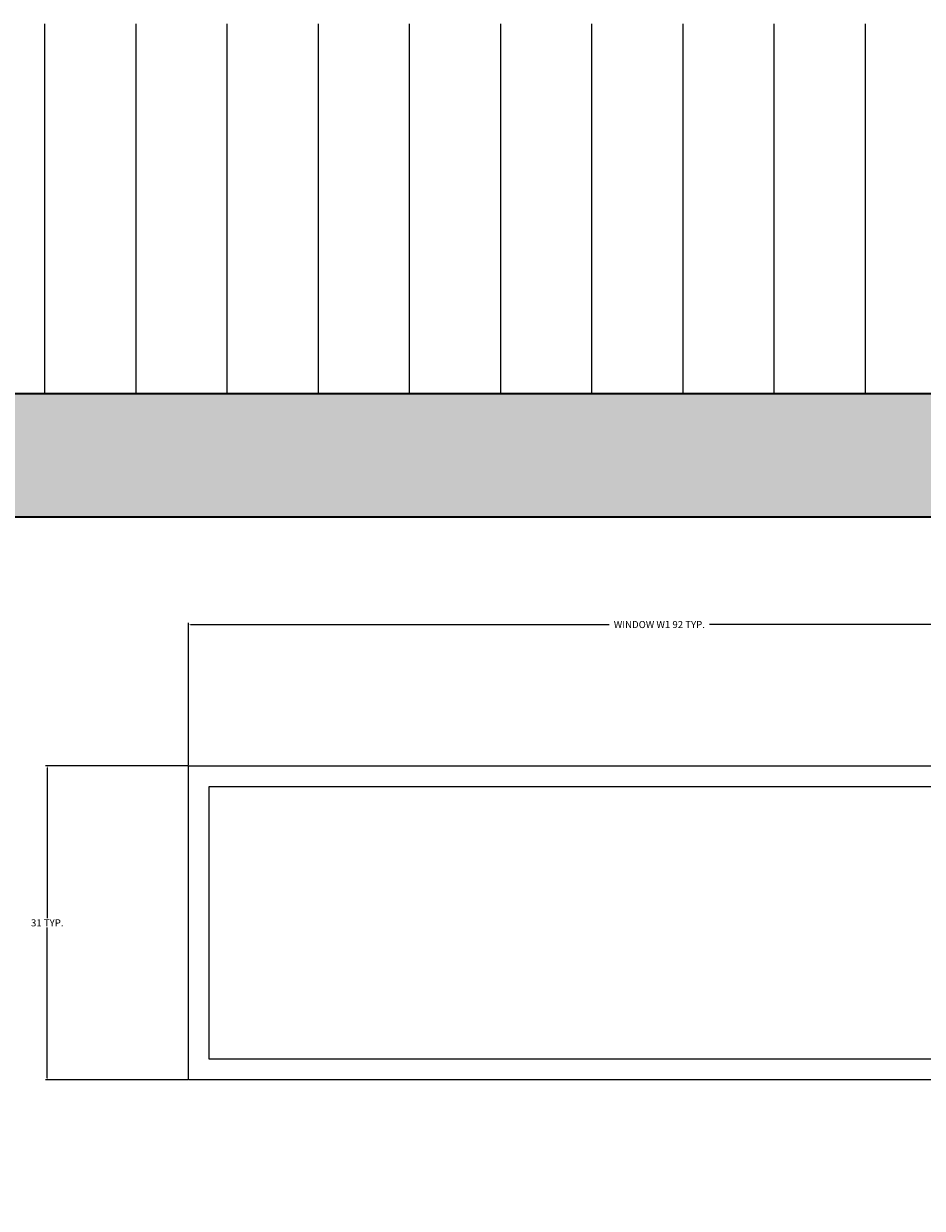
# Model space of a CAD drawing. Units: inches. Extents: x -145 to 510, y 5 to 386.
# Tile 23 of 25: x 335 to 423, y 157 to 272. Entities that reach past the tile are written whole.
import ezdxf

# ---------------------------------------------------------------- set-up
doc = ezdxf.new("R2010")
doc.units = ezdxf.units.IN
doc.header["$MEASUREMENT"] = 0
for name, color, linetype, lineweight in [('A-ANNO-DIMS', 2, 'Continuous', 18), ('A-ELEV', 7, 'Continuous', 35), ('A-ELEV-PATT', 8, 'Continuous', 13), ('A-GLAZ', 4, 'Continuous', 25)]:
    doc.layers.add(name, color=color, linetype=linetype, lineweight=lineweight)
doc.styles.get("Standard").update_dxf_attribs({"font": 'arial.ttf'})
doc.dimstyles.get("Standard").update_dxf_attribs({"dimtxt": 0.6875, "dimasz": 0.18, "dimexe": 0.18, "dimexo": 0.0625, "dimgap": 0.09, "dimtad": 0, "dimtih": 1, "dimtoh": 1, "dimdec": 4, "dimzin": 0, "dimdsep": 46, "dimlunit": 4, "dimtxsty": 'Standard', "dimcen": 0.09, "dimadec": 0, "dimazin": 0, "dimtfac": 1, "dimtdec": 4, "dimtofl": 0, "dimtmove": 0, "dimatfit": 3, "dimfxl": 1, "dimtolj": 1, "dimtzin": 0, "dimarcsym": 0})

# ---------------------------------------------------------------- blocks, each defined once
blk = doc.blocks.new('WIN-2200')
for points in [[(0, 30.55), (91.67, 30.55), (91.67, 0), (0, 0)], [(2, 28.55), (89.67, 28.55), (89.67, 2), (2, 2)]]:
    blk.add_lwpolyline(points, close=True)
blk = doc.blocks.new('*D5')
at = {"layer": 'A-ANNO-DIMS', "color": 0, "lineweight": -2, "transparency": 16777216}
for p, q in [((351.23, 199.73), (351.23, 213.6)), ((351.41, 213.42), (392.2, 213.42)), ((442.72, 213.42), (401.94, 213.42)), ((442.9, 199.73), (442.9, 213.6))]:
    blk.add_line(p, q, dxfattribs=at)
at = {"layer": 'A-ANNO-DIMS', "color": 0, "transparency": 16777216}
for points in [[(351.41, 213.45), (351.41, 213.39), (351.23, 213.42)], [(442.72, 213.45), (442.72, 213.39), (442.9, 213.42)]]:
    blk.add_solid(points, dxfattribs=at)
at = {"layer": 'Defpoints', "color": 0, "transparency": 16777216}
for p in [(442.9, 213.42), (351.23, 199.67), (442.9, 199.67)]:
    blk.add_point(p, dxfattribs=at)
at = {"layer": 'A-ANNO-DIMS', "color": 0, "transparency": 16777216, "insert": (397.07, 213.42), "char_height": 0.6875, "attachment_point": 5}
blk.add_mtext('\\A1;WINDOW W1 92 TYP.', dxfattribs=at)
blk = doc.blocks.new('*D6')
at = {"layer": 'A-ANNO-DIMS', "color": 0, "lineweight": -2, "transparency": 16777216}
for p, q in [((351.17, 199.67), (337.3, 199.67)), ((337.48, 199.49), (337.48, 184.83)), ((337.48, 169.29), (337.48, 183.95)), ((351.17, 169.11), (337.3, 169.11))]:
    blk.add_line(p, q, dxfattribs=at)
at = {"layer": 'A-ANNO-DIMS', "color": 0, "transparency": 16777216}
for points in [[(337.45, 199.49), (337.51, 199.49), (337.48, 199.67)], [(337.45, 169.29), (337.51, 169.29), (337.48, 169.11)]]:
    blk.add_solid(points, dxfattribs=at)
at = {"layer": 'Defpoints', "color": 0, "transparency": 16777216}
for p in [(337.48, 199.67), (351.23, 199.67), (351.23, 169.11)]:
    blk.add_point(p, dxfattribs=at)
at = {"layer": 'A-ANNO-DIMS', "color": 0, "transparency": 16777216, "insert": (337.48, 184.39), "char_height": 0.6875, "attachment_point": 5}
blk.add_mtext('\\A1;31 TYP.', dxfattribs=at)
blk = doc.blocks.new('*D19')
at = {"layer": 'A-ANNO-DIMS', "color": 0, "lineweight": -2, "transparency": 16777216}
for p, q in [((478.76, 355.89), (-144.05, 355.89)), ((-143.87, 355.71), (-143.87, 218.33)), ((-143.87, 80.07), (-143.87, 217.45)), ((-114.04, 79.89), (-144.05, 79.89))]:
    blk.add_line(p, q, dxfattribs=at)
at = {"layer": 'A-ANNO-DIMS', "color": 0, "transparency": 16777216}
for points in [[(-143.9, 355.71), (-143.84, 355.71), (-143.87, 355.89)], [(-143.9, 80.07), (-143.84, 80.07), (-143.87, 79.89)]]:
    blk.add_solid(points, dxfattribs=at)
at = {"layer": 'Defpoints', "color": 0, "transparency": 16777216}
for p in [(-143.87, 355.89), (478.83, 355.89), (-113.97, 79.89)]:
    blk.add_point(p, dxfattribs=at)
at = {"layer": 'A-ANNO-DIMS', "color": 0, "transparency": 16777216, "insert": (-143.87, 217.89), "char_height": 0.688, "attachment_point": 5}
blk.add_mtext('\\A1;276', dxfattribs=at)

msp = doc.modelspace()

# ---------------------------------------------------------------- hatches: boundary and pattern name
at = {"layer": 'A-ELEV-PATT'}
h = msp.add_hatch(color=256, dxfattribs=at)
h.dxf.hatch_style = 1
h.paths.add_polyline_path([(334.4402, 341.168), (69.7763, 341.168), (69.7763, 327.6093), (334.4402, 327.6093)])
h.paths.add_polyline_path([(69.7763, 341.168), (34.2706, 341.168), (34.2706, 327.6093), (69.7763, 327.6093)])
h.paths.add_polyline_path([(317.2273, 188.3087), (210.7973, 188.3087), (210.7973, 178.0195), (317.2273, 178.0195)])
h.paths.add_polyline_path([(474.4893, 235.8905), (317.2273, 235.8905), (317.2273, 223.8905), (474.4893, 223.8905)])
h.paths.add_polyline_path([(317.2273, 235.8905), (309.4739, 235.8905), (309.4739, 223.8905), (317.2273, 223.8905)])
h.paths.add_polyline_path([(478.8263, 235.8905), (474.4893, 235.8905), (474.4893, 223.8905), (478.8263, 223.8905)])
h = msp.add_hatch(dxfattribs=at)
h.set_pattern_fill('ANSI31', color=256, scale=71, angle=45)
h.paths.add_polyline_path([(478.8263, 271.8905), (309.4739, 271.8905), (309.4739, 259.8905), (309.4739, 235.8905), (317.2273, 235.8905), (474.4893, 235.8905), (478.8263, 235.8905)])

# ---------------------------------------------------------------- linework, layer by layer
at = {"layer": 'A-ELEV'}
for p, q in [((317.2273, 235.8905), (474.4893, 235.8905)), ((317.2273, 223.8905), (474.4893, 223.8905))]:
    msp.add_line(p, q, dxfattribs=at)

# ---------------------------------------------------------------- block references
at = {"layer": 'A-GLAZ'}
msp.add_blockref('WIN-2200', (351.234, 169.112), dxfattribs=at)

# ---------------------------------------------------------------- dimensions: what is measured, and where the dimension line sits
at = {"layer": 'A-ANNO-DIMS'}
dim = msp.add_linear_dim(base=(-143.8737, 355.8905), p1=(-113.9737, 79.8905), p2=(478.8263, 355.8905), angle=90, dimstyle='Standard', override={"dimdec": 0, "dimlfac": 1, "dimrnd": 0, "dimzin": 0, "dimdsep": 46, "dimlunit": 2}, dxfattribs=at)
dim.commit()
dim.dimension.update_dxf_attribs({"geometry": '*D19', "text_midpoint": (-143.8737, 217.8905)})
dim = msp.add_linear_dim(base=(442.9009, 213.4154), p1=(351.234, 199.6654), p2=(442.9009, 199.6654), text='WINDOW W1 <> TYP.', dimstyle='Standard', override={"dimdec": 0, "dimlfac": 1, "dimrnd": 0, "dimzin": 0, "dimdsep": 46, "dimlunit": 2}, dxfattribs=at)
dim.commit()
dim.dimension.update_dxf_attribs({"geometry": '*D5', "text_midpoint": (397.0675, 213.4154)})
dim = msp.add_linear_dim(base=(337.484, 199.6654), p1=(351.234, 169.1117), p2=(351.234, 199.6654), angle=90, text='<> TYP.', dimstyle='Standard', override={"dimdec": 0, "dimlfac": 1, "dimrnd": 0, "dimzin": 0, "dimdsep": 46, "dimlunit": 2}, dxfattribs=at)
dim.commit()
dim.dimension.update_dxf_attribs({"geometry": '*D6', "text_midpoint": (337.484, 184.3886)})

doc.saveas('drawing.dxf')
